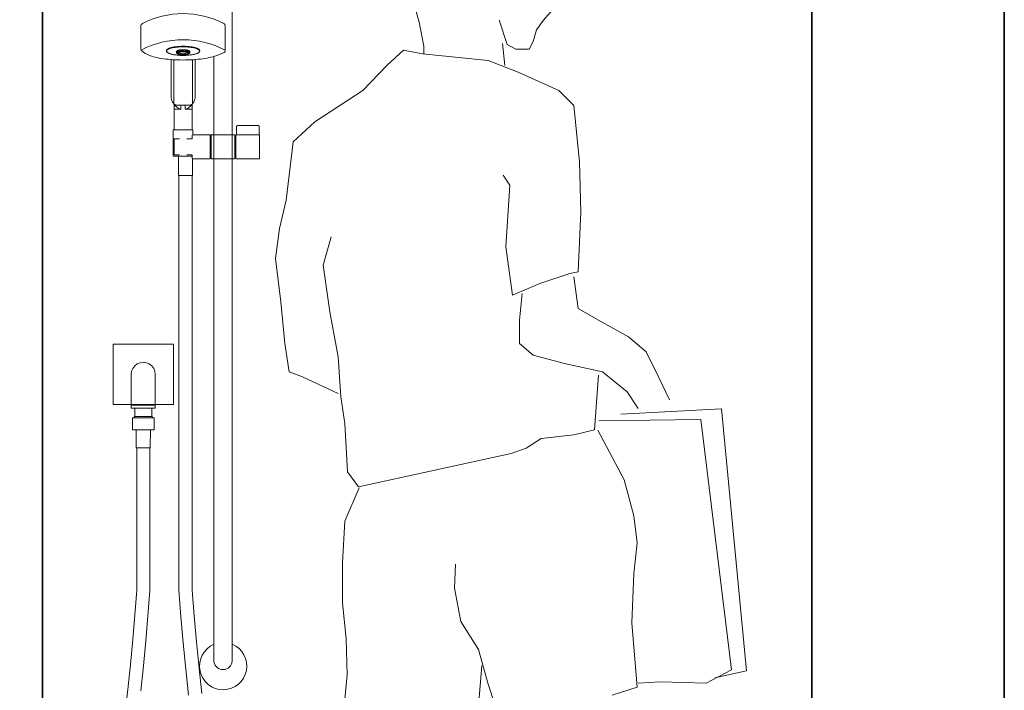
# Model space of a CAD drawing. Units: inches. Extents: x 64 to 1167, y 117 to 939.
# Tile 39 of 56: x 1121 to 1167, y 464 to 496. Entities that reach past the tile are written whole.
import ezdxf

# ---------------------------------------------------------------- set-up
doc = ezdxf.new("R2010")
doc.units = ezdxf.units.IN
doc.header["$MEASUREMENT"] = 0
for name, color, linetype, lineweight in [('A-ENTG', 8, 'Continuous', 18), ('A-FLOR-FIXT', 8, 'Continuous', 18), ('A-SECT', 7, 'Continuous', 35)]:
    doc.layers.add(name, color=color, linetype=linetype, lineweight=lineweight)

# ---------------------------------------------------------------- blocks, each defined once
blk = doc.blocks.new('A$C43851DCA')
at = {"linetype": 'ByBlock'}
for p, q in [((0.0065, 0.059624), (0.006721, 0.058807)), ((0.013179, 0.059624), (0.012552, 0.058897)), ((0.006721, 0.058807), (0.006948, 0.057674)), ((0.010844, 0.057764), (0.01047, 0.058897)), ((0.012552, 0.058897), (0.012215, 0.058446)), ((0.012215, 0.058446), (0.012067, 0.057905)), ((0.006948, 0.057674), (0.006948, 0.057313)), ((0.010733, 0.056772), (0.010623, 0.057809)), ((0.01125, 0.057538), (0.010844, 0.057764)), ((0.012067, 0.057905), (0.011882, 0.057538)), ((0.005999, 0.057487), (0.00523, 0.056785)), ((0.00689, 0.057326), (0.005999, 0.057487)), ((0.009953, 0.057017), (0.00689, 0.057326)), ((0.011882, 0.057538), (0.01125, 0.057538)), ((0.00523, 0.056785), (0.004086, 0.055614)), ((0.011355, 0.05647), (0.009953, 0.057017)), ((0.013269, 0.055614), (0.011355, 0.05647)), ((0.004086, 0.055614), (0.00185, 0.054133)), ((0.01397, 0.054912), (0.013269, 0.055614)), ((0.014223, 0.052266), (0.01397, 0.054912)), ((0.00185, 0.054133), (0.000828, 0.053199)), ((0.000828, 0.053199), (0.000511, 0.050476)), ((0.014292, 0.049929), (0.014223, 0.052266)), ((0.010654, 0.051642), (0.01097, 0.051172)), ((0.01097, 0.051172), (0.010781, 0.048294)), ((0.000511, 0.050476), (0.00019, 0.04915)), ((0.01416, 0.047122), (0.014292, 0.049929)), ((0.00019, 0.04915), (0, 0.047747)), ((0.002615, 0.048758), (0.002235, 0.047438)), ((0.010781, 0.048294), (0.011102, 0.046035)), ((0, 0.047747), (0.000258, 0.045726)), ((0.002235, 0.047438), (0.002552, 0.045256)), ((0.012378, 0.046582), (0.01378, 0.047045)), ((0.01378, 0.047045), (0.01416, 0.047122)), ((0.011102, 0.046035), (0.012378, 0.046582)), ((0.01397, 0.046891), (0.01416, 0.04541)), ((0.011545, 0.046112), (0.011419, 0.044863)), ((0.000258, 0.045726), (0.000448, 0.043775)), ((0.002552, 0.045256), (0.002936, 0.043151)), ((0.01416, 0.04541), (0.015119, 0.044863)), ((0.011419, 0.044863), (0.011419, 0.043775)), ((0.015119, 0.044863), (0.016522, 0.044084)), ((0.000448, 0.043775), (0.000638, 0.042449)), ((0.011419, 0.043775), (0.012056, 0.043228)), ((0.016522, 0.044084), (0.017349, 0.043389)), ((0.017349, 0.043389), (0.017924, 0.042217)), ((0.002936, 0.043151), (0.003063, 0.041284)), ((0.012056, 0.043228), (0.013522, 0.042842)), ((0.000638, 0.042449), (0.001276, 0.042217)), ((0.013522, 0.042842), (0.015309, 0.042449)), ((0.015309, 0.042449), (0.016458, 0.041515)), ((0.001276, 0.042217), (0.002936, 0.041438)), ((0.014929, 0.039726), (0.015119, 0.042294)), ((0.017924, 0.042217), (0.018435, 0.041129)), ((0.016458, 0.041515), (0.01697, 0.040736)), ((0.003063, 0.041284), (0.003253, 0.040035)), ((0.020871, 0.040711), (0.016163, 0.04046)), ((0.022052, 0.028454), (0.020871, 0.040711)), ((0.015135, 0.040151), (0.019901, 0.040209)), ((0.019901, 0.040209), (0.021335, 0.028512)), ((0.003253, 0.040035), (0.003379, 0.037775)), ((0.01397, 0.039494), (0.014929, 0.039726)), ((0.016316, 0.037395), (0.015082, 0.039713)), ((0.01174, 0.03887), (0.012441, 0.039333)), ((0.012441, 0.039333), (0.01397, 0.039494)), ((0.011034, 0.038631), (0.01174, 0.03887)), ((0.003891, 0.037074), (0.011034, 0.038631)), ((0.003379, 0.037775), (0.003891, 0.037074)), ((0.016775, 0.035709), (0.016316, 0.037395)), ((0.003917, 0.037022), (0.003253, 0.035458)), ((0.016927, 0.034453), (0.016775, 0.035709)), ((0.003253, 0.035458), (0.003147, 0.03352)), ((0.016775, 0.033018), (0.016927, 0.034453)), ((0.003147, 0.03352), (0.003147, 0.03164)), ((0.008424, 0.033456), (0.008377, 0.032329)), ((0.016674, 0.030707), (0.016775, 0.033018)), ((0.008377, 0.032329), (0.008683, 0.030765)), ((0.003147, 0.03164), (0.003305, 0.029954)), ((0.008683, 0.030765), (0.0095, 0.029452)), ((0.016927, 0.027701), (0.016674, 0.030707)), ((0.003305, 0.029954), (0.003353, 0.028267)), ((0.0095, 0.029452), (0.009964, 0.027829)), ((0.0095, 0.026825), (0.009658, 0.028705)), ((0.003353, 0.028267), (0.003253, 0.02714)), ((0.021335, 0.028512), (0.020154, 0.027887)), ((0.020565, 0.028138), (0.022052, 0.028454)), ((0.009964, 0.027829), (0.010269, 0.026889)), ((0.015752, 0.027327), (0.016927, 0.027701)), ((0.018003, 0.027952), (0.01698, 0.027887)), ((0.020154, 0.027887), (0.018003, 0.027952))]:
    blk.add_line(p, q, dxfattribs=at)

msp = doc.modelspace()

# ---------------------------------------------------------------- linework, layer by layer
at = {"layer": 'A-FLOR-FIXT'}
for p, q in [((1130.678, 499.898), (1130.678, 490.219)), ((1126.411, 494.238), (1126.411, 495.296)), ((1130.362, 494.172), (1130.362, 495.296)), ((1126.615, 494.023), (1126.467, 494.13)), ((1126.663, 493.994), (1126.615, 494.023)), ((1126.717, 493.967), (1126.663, 493.994)), ((1126.778, 493.94), (1126.717, 493.967)), ((1126.845, 493.914), (1126.778, 493.94)), ((1126.919, 493.89), (1126.845, 493.914)), ((1127.61, 494.153), (1127.612, 494.166)), ((1127.612, 494.141), (1127.61, 494.153)), ((1127.61, 494.128), (1127.612, 494.141)), ((1127.612, 494.115), (1127.61, 494.128)), ((1127.612, 494.166), (1127.616, 494.178)), ((1127.612, 494.141), (1127.616, 494.153)), ((1127.616, 494.102), (1127.612, 494.115)), ((1127.616, 494.178), (1127.624, 494.191)), ((1127.616, 494.153), (1127.624, 494.165)), ((1127.624, 494.09), (1127.616, 494.102)), ((1127.624, 494.191), (1127.635, 494.203)), ((1127.624, 494.165), (1127.635, 494.178)), ((1127.635, 494.078), (1127.624, 494.09)), ((1127.635, 494.103), (1127.625, 494.115)), ((1127.635, 494.203), (1127.648, 494.215)), ((1127.635, 494.178), (1127.648, 494.19)), ((1127.648, 494.091), (1127.635, 494.103)), ((1127.648, 494.066), (1127.635, 494.078)), ((1127.648, 494.215), (1127.665, 494.227)), ((1127.648, 494.19), (1127.665, 494.202)), ((1127.649, 494.09), (1127.648, 494.091)), ((1127.665, 494.054), (1127.648, 494.066)), ((1127.665, 494.227), (1127.684, 494.239)), ((1127.665, 494.202), (1127.684, 494.213)), ((1127.684, 494.042), (1127.665, 494.054)), ((1127.684, 494.239), (1127.706, 494.25)), ((1127.684, 494.213), (1127.706, 494.224)), ((1127.706, 494.031), (1127.684, 494.042)), ((1127.706, 494.25), (1127.731, 494.261)), ((1127.706, 494.224), (1127.731, 494.235)), ((1127.731, 494.02), (1127.706, 494.031)), ((1127.731, 494.261), (1127.759, 494.271)), ((1127.731, 494.235), (1127.759, 494.246)), ((1127.759, 494.01), (1127.731, 494.02)), ((1127.759, 494.271), (1127.788, 494.281)), ((1127.759, 494.246), (1127.788, 494.256)), ((1127.788, 494), (1127.759, 494.01)), ((1127.788, 494.281), (1127.821, 494.291)), ((1127.788, 494.256), (1127.821, 494.265)), ((1127.821, 493.99), (1127.788, 494)), ((1127.821, 494.291), (1127.855, 494.3)), ((1127.821, 494.265), (1127.855, 494.274)), ((1127.855, 493.981), (1127.821, 493.99)), ((1127.855, 494.3), (1127.892, 494.308)), ((1127.855, 494.274), (1127.892, 494.282)), ((1127.892, 493.973), (1127.855, 493.981)), ((1127.892, 494.308), (1127.93, 494.316)), ((1127.892, 494.282), (1127.93, 494.29)), ((1127.93, 493.965), (1127.892, 493.973)), ((1127.93, 494.316), (1127.971, 494.323)), ((1127.93, 494.29), (1127.971, 494.297)), ((1127.971, 493.958), (1127.93, 493.965)), ((1127.971, 494.323), (1128.013, 494.329)), ((1127.971, 494.297), (1128.013, 494.304)), ((1128.013, 493.952), (1127.971, 493.958)), ((1128.013, 494.329), (1128.056, 494.335)), ((1128.013, 494.304), (1128.056, 494.309)), ((1128.056, 493.946), (1128.013, 493.952)), ((1128.056, 494.335), (1128.101, 494.34)), ((1128.056, 494.309), (1128.101, 494.314)), ((1128.101, 493.941), (1128.056, 493.946)), ((1128.076, 494.112), (1128.077, 494.117)), ((1128.077, 494.107), (1128.076, 494.112)), ((1128.077, 494.049), (1128.076, 494.044)), ((1128.076, 494.044), (1128.077, 494.039)), ((1128.077, 494.117), (1128.079, 494.122)), ((1128.079, 494.102), (1128.077, 494.107)), ((1128.079, 494.054), (1128.077, 494.049)), ((1128.077, 494.039), (1128.079, 494.034)), ((1128.079, 494.122), (1128.082, 494.127)), ((1128.079, 494.054), (1128.079, 494.102)), ((1128.082, 494.059), (1128.079, 494.054)), ((1128.079, 494.034), (1128.082, 494.029)), ((1128.082, 494.127), (1128.086, 494.132)), ((1128.086, 494.092), (1128.082, 494.097)), ((1128.086, 494.064), (1128.082, 494.059)), ((1128.082, 494.029), (1128.086, 494.024)), ((1128.086, 494.132), (1128.091, 494.137)), ((1128.091, 494.087), (1128.086, 494.092)), ((1128.091, 494.069), (1128.086, 494.064)), ((1128.086, 494.024), (1128.091, 494.019)), ((1128.091, 494.137), (1128.098, 494.142)), ((1128.098, 494.083), (1128.091, 494.087)), ((1128.091, 494.069), (1128.098, 494.074)), ((1128.091, 494.019), (1128.098, 494.015)), ((1128.098, 494.142), (1128.106, 494.146)), ((1128.106, 494.078), (1128.098, 494.083)), ((1128.098, 494.074), (1128.106, 494.078)), ((1128.098, 494.015), (1128.106, 494.01)), ((1128.101, 494.34), (1128.147, 494.344)), ((1128.101, 494.314), (1128.147, 494.319)), ((1128.147, 493.937), (1128.101, 493.941)), ((1128.106, 494.146), (1128.114, 494.151)), ((1128.106, 494.078), (1128.111, 494.081)), ((1128.111, 494.075), (1128.106, 494.078)), ((1128.106, 494.01), (1128.114, 494.005)), ((1128.111, 494.081), (1128.114, 494.083)), ((1128.111, 494.081), (1128.111, 494.075)), ((1128.114, 494.074), (1128.111, 494.075)), ((1128.111, 494.075), (1128.111, 494.062)), ((1128.111, 494.058), (1128.114, 494.053)), ((1128.111, 494.044), (1128.112, 494.049)), ((1128.112, 494.04), (1128.111, 494.044)), ((1128.112, 494.049), (1128.114, 494.053)), ((1128.114, 494.035), (1128.112, 494.04)), ((1128.114, 494.151), (1128.124, 494.155)), ((1128.116, 494.126), (1128.114, 494.123)), ((1128.116, 494.115), (1128.114, 494.112)), ((1128.114, 494.092), (1128.116, 494.089)), ((1128.114, 494.083), (1128.12, 494.084)), ((1128.124, 494.069), (1128.114, 494.074)), ((1128.114, 494.053), (1128.116, 494.057)), ((1128.116, 494.031), (1128.114, 494.035)), ((1128.114, 494.005), (1128.124, 494.001)), ((1128.12, 494.13), (1128.116, 494.126)), ((1128.12, 494.12), (1128.116, 494.115)), ((1128.116, 494.089), (1128.12, 494.084)), ((1128.116, 494.057), (1128.12, 494.062)), ((1128.12, 494.026), (1128.116, 494.031)), ((1128.125, 494.134), (1128.12, 494.13)), ((1128.125, 494.124), (1128.12, 494.12)), ((1128.12, 494.084), (1128.124, 494.087)), ((1128.12, 494.084), (1128.125, 494.08)), ((1128.12, 494.062), (1128.125, 494.066)), ((1128.125, 494.022), (1128.12, 494.026)), ((1128.124, 494.155), (1128.135, 494.159)), ((1128.124, 494.087), (1128.135, 494.091)), ((1128.127, 494.068), (1128.124, 494.069)), ((1128.124, 494.001), (1128.135, 493.997)), ((1128.131, 494.138), (1128.125, 494.134)), ((1128.131, 494.128), (1128.125, 494.124)), ((1128.125, 494.08), (1128.131, 494.076)), ((1128.125, 494.066), (1128.127, 494.068)), ((1128.131, 494.018), (1128.125, 494.022)), ((1128.127, 494.068), (1128.131, 494.07)), ((1128.135, 494.065), (1128.127, 494.068)), ((1128.135, 494.141), (1128.131, 494.138)), ((1128.135, 494.131), (1128.131, 494.128)), ((1128.131, 494.076), (1128.135, 494.073)), ((1128.131, 494.07), (1128.135, 494.073)), ((1128.138, 494.014), (1128.131, 494.018)), ((1128.135, 494.159), (1128.147, 494.163)), ((1128.135, 494.091), (1128.147, 494.095)), ((1128.135, 494.073), (1128.138, 494.074)), ((1128.135, 494.073), (1128.138, 494.072)), ((1128.138, 494.064), (1128.135, 494.065)), ((1128.135, 493.997), (1128.147, 493.993)), ((1128.138, 494.074), (1128.145, 494.078)), ((1128.138, 494.072), (1128.145, 494.068)), ((1128.145, 494.01), (1128.138, 494.014)), ((1128.145, 494.078), (1128.154, 494.082)), ((1128.145, 494.068), (1128.154, 494.064)), ((1128.147, 494.061), (1128.145, 494.062)), ((1128.154, 494.006), (1128.145, 494.01)), ((1128.147, 494.344), (1128.193, 494.348)), ((1128.147, 494.319), (1128.193, 494.322)), ((1128.147, 494.163), (1128.16, 494.167)), ((1128.154, 494.15), (1128.147, 494.147)), ((1128.154, 494.14), (1128.147, 494.137)), ((1128.16, 494.099), (1128.147, 494.095)), ((1128.16, 494.057), (1128.147, 494.061)), ((1128.147, 493.993), (1128.16, 493.989)), ((1128.193, 493.933), (1128.147, 493.937)), ((1128.16, 494.153), (1128.154, 494.15)), ((1128.16, 494.142), (1128.154, 494.14)), ((1128.154, 494.082), (1128.164, 494.086)), ((1128.154, 494.064), (1128.164, 494.06)), ((1128.164, 494.002), (1128.154, 494.006)), ((1128.16, 494.167), (1128.174, 494.171)), ((1128.174, 494.103), (1128.16, 494.099)), ((1128.164, 494.056), (1128.16, 494.057)), ((1128.16, 493.989), (1128.174, 493.986)), ((1128.164, 494.086), (1128.174, 494.089)), ((1128.164, 494.06), (1128.174, 494.057)), ((1128.174, 493.999), (1128.164, 494.002)), ((1128.174, 494.171), (1128.189, 494.174)), ((1128.186, 494.161), (1128.174, 494.158)), ((1128.186, 494.151), (1128.174, 494.147)), ((1128.189, 494.106), (1128.174, 494.103)), ((1128.174, 494.089), (1128.186, 494.093)), ((1128.174, 494.057), (1128.186, 494.053)), ((1128.186, 494.051), (1128.174, 494.054)), ((1128.186, 493.995), (1128.174, 493.999)), ((1128.174, 493.986), (1128.189, 493.982)), ((1128.189, 494.162), (1128.186, 494.161)), ((1128.189, 494.151), (1128.186, 494.151)), ((1128.186, 494.093), (1128.198, 494.096)), ((1128.186, 494.053), (1128.198, 494.05)), ((1128.198, 493.992), (1128.186, 493.995)), ((1128.189, 494.174), (1128.204, 494.177)), ((1128.204, 494.109), (1128.189, 494.106)), ((1128.189, 493.982), (1128.204, 493.979)), ((1128.193, 494.348), (1128.241, 494.35)), ((1128.193, 494.322), (1128.241, 494.325)), ((1128.241, 493.93), (1128.193, 493.933)), ((1128.198, 494.096), (1128.211, 494.099)), ((1128.198, 494.05), (1128.204, 494.047)), ((1128.204, 494.047), (1128.198, 494.048)), ((1128.211, 493.989), (1128.198, 493.992)), ((1128.204, 494.177), (1128.22, 494.18)), ((1128.211, 494.167), (1128.204, 494.165)), ((1128.211, 494.157), (1128.204, 494.155)), ((1128.22, 494.112), (1128.204, 494.109)), ((1128.204, 494.047), (1128.211, 494.047)), ((1128.204, 493.979), (1128.22, 493.976)), ((1128.22, 494.169), (1128.211, 494.167)), ((1128.22, 494.159), (1128.211, 494.157)), ((1128.211, 494.099), (1128.225, 494.102)), ((1128.211, 494.047), (1128.22, 494.044)), ((1128.225, 493.986), (1128.211, 493.989)), ((1128.22, 494.18), (1128.237, 494.183)), ((1128.237, 494.114), (1128.22, 494.112)), ((1128.225, 494.044), (1128.22, 494.044)), ((1128.22, 493.976), (1128.237, 493.974)), ((1128.225, 494.102), (1128.239, 494.104)), ((1128.225, 494.044), (1128.239, 494.042)), ((1128.239, 493.984), (1128.225, 493.986)), ((1128.237, 494.183), (1128.254, 494.185)), ((1128.254, 494.117), (1128.237, 494.114)), ((1128.237, 493.974), (1128.254, 493.971)), ((1128.239, 494.104), (1128.254, 494.106)), ((1128.239, 494.042), (1128.254, 494.04)), ((1128.254, 493.982), (1128.239, 493.984)), ((1128.241, 494.35), (1128.289, 494.352)), ((1128.241, 494.325), (1128.289, 494.327)), ((1128.289, 493.928), (1128.241, 493.93)), ((1128.254, 494.185), (1128.272, 494.187)), ((1128.269, 494.177), (1128.254, 494.175)), ((1128.269, 494.166), (1128.254, 494.164)), ((1128.272, 494.119), (1128.254, 494.117)), ((1128.254, 494.106), (1128.269, 494.109)), ((1128.254, 494.04), (1128.269, 494.038)), ((1128.269, 493.98), (1128.254, 493.982)), ((1128.254, 493.971), (1128.272, 493.969)), ((1128.272, 494.177), (1128.269, 494.177)), ((1128.272, 494.167), (1128.269, 494.166)), ((1128.269, 494.109), (1128.285, 494.11)), ((1128.269, 494.038), (1128.285, 494.036)), ((1128.285, 493.978), (1128.269, 493.98)), ((1128.272, 494.187), (1128.291, 494.189)), ((1128.291, 494.12), (1128.272, 494.119)), ((1128.272, 493.969), (1128.291, 493.968)), ((1128.285, 494.11), (1128.301, 494.112)), ((1128.285, 494.036), (1128.301, 494.034)), ((1128.301, 493.976), (1128.285, 493.978)), ((1128.289, 494.352), (1128.338, 494.354)), ((1128.289, 494.327), (1128.338, 494.328)), ((1128.338, 493.927), (1128.289, 493.928)), ((1128.291, 494.189), (1128.309, 494.19)), ((1128.301, 494.18), (1128.291, 494.179)), ((1128.301, 494.17), (1128.291, 494.169)), ((1128.309, 494.122), (1128.291, 494.12)), ((1128.291, 493.968), (1128.309, 493.966)), ((1128.309, 494.181), (1128.301, 494.18)), ((1128.309, 494.17), (1128.301, 494.17)), ((1128.301, 494.112), (1128.318, 494.113)), ((1128.301, 494.034), (1128.318, 494.033)), ((1128.318, 493.975), (1128.301, 493.976)), ((1128.309, 494.19), (1128.328, 494.191)), ((1128.328, 494.123), (1128.309, 494.122)), ((1128.309, 493.966), (1128.328, 493.965)), ((1128.318, 494.113), (1128.335, 494.114)), ((1128.318, 494.033), (1128.335, 494.032)), ((1128.335, 493.974), (1128.318, 493.975)), ((1128.328, 494.191), (1128.348, 494.192)), ((1128.348, 494.124), (1128.328, 494.123)), ((1128.328, 493.965), (1128.348, 493.964)), ((1128.335, 494.114), (1128.352, 494.115)), ((1128.335, 494.032), (1128.352, 494.031)), ((1128.352, 493.973), (1128.335, 493.974)), ((1128.338, 494.354), (1128.386, 494.354)), ((1128.338, 494.328), (1128.386, 494.328)), ((1128.386, 493.927), (1128.338, 493.927)), ((1128.348, 494.192), (1128.367, 494.192)), ((1128.352, 494.183), (1128.348, 494.183)), ((1128.352, 494.173), (1128.348, 494.172)), ((1128.367, 494.124), (1128.348, 494.124)), ((1128.348, 493.964), (1128.367, 493.964)), ((1128.367, 494.183), (1128.352, 494.183)), ((1128.367, 494.173), (1128.352, 494.173)), ((1128.352, 494.115), (1128.369, 494.115)), ((1128.352, 494.031), (1128.369, 494.031)), ((1128.369, 493.973), (1128.352, 493.973)), ((1128.367, 494.192), (1128.386, 494.193)), ((1128.386, 494.124), (1128.367, 494.124)), ((1128.367, 493.964), (1128.386, 493.964)), ((1128.369, 494.115), (1128.386, 494.115)), ((1128.369, 494.031), (1128.386, 494.031)), ((1128.386, 493.973), (1128.369, 493.973)), ((1128.386, 494.354), (1128.435, 494.354)), ((1128.386, 494.328), (1128.435, 494.328)), ((1128.386, 494.193), (1128.406, 494.192)), ((1128.406, 494.124), (1128.386, 494.124)), ((1128.386, 494.115), (1128.404, 494.115)), ((1128.386, 494.031), (1128.404, 494.031)), ((1128.404, 493.973), (1128.386, 493.973)), ((1128.386, 493.964), (1128.406, 493.964)), ((1128.435, 493.927), (1128.386, 493.927)), ((1128.404, 494.115), (1128.421, 494.115)), ((1128.404, 494.031), (1128.421, 494.031)), ((1128.421, 493.973), (1128.404, 493.973)), ((1128.406, 494.192), (1128.425, 494.192)), ((1128.421, 494.183), (1128.406, 494.183)), ((1128.421, 494.173), (1128.406, 494.173)), ((1128.425, 494.124), (1128.406, 494.124)), ((1128.406, 493.964), (1128.425, 493.964)), ((1128.425, 494.183), (1128.421, 494.183)), ((1128.425, 494.172), (1128.421, 494.173)), ((1128.421, 494.115), (1128.438, 494.114)), ((1128.421, 494.031), (1128.438, 494.032)), ((1128.438, 493.974), (1128.421, 493.973)), ((1128.425, 494.192), (1128.445, 494.191)), ((1128.445, 494.123), (1128.425, 494.124)), ((1128.425, 493.964), (1128.445, 493.965)), ((1128.435, 494.354), (1128.484, 494.352)), ((1128.435, 494.328), (1128.484, 494.327)), ((1128.484, 493.928), (1128.435, 493.927)), ((1128.438, 494.114), (1128.455, 494.113)), ((1128.438, 494.032), (1128.455, 494.033)), ((1128.455, 493.975), (1128.438, 493.974)), ((1128.445, 494.191), (1128.464, 494.19)), ((1128.464, 494.122), (1128.445, 494.123)), ((1128.445, 493.965), (1128.464, 493.966)), ((1128.455, 494.113), (1128.471, 494.112)), ((1128.455, 494.033), (1128.471, 494.034)), ((1128.471, 493.976), (1128.455, 493.975)), ((1128.464, 494.19), (1128.482, 494.189)), ((1128.471, 494.18), (1128.464, 494.181)), ((1128.471, 494.17), (1128.464, 494.17)), ((1128.464, 494.122), (1128.482, 494.12)), ((1128.464, 493.966), (1128.482, 493.968)), ((1128.482, 494.179), (1128.471, 494.18)), ((1128.482, 494.169), (1128.471, 494.17)), ((1128.471, 494.112), (1128.488, 494.11)), ((1128.471, 494.034), (1128.488, 494.036)), ((1128.488, 493.978), (1128.471, 493.976)), ((1128.482, 494.189), (1128.501, 494.187)), ((1128.482, 494.12), (1128.501, 494.119)), ((1128.482, 493.968), (1128.501, 493.969)), ((1128.484, 494.352), (1128.532, 494.35)), ((1128.484, 494.327), (1128.532, 494.325)), ((1128.532, 493.93), (1128.484, 493.928)), ((1128.488, 494.11), (1128.504, 494.109)), ((1128.488, 494.036), (1128.504, 494.038)), ((1128.504, 493.98), (1128.488, 493.978)), ((1128.501, 494.187), (1128.519, 494.185)), ((1128.501, 494.119), (1128.519, 494.117)), ((1128.501, 493.969), (1128.519, 493.971)), ((1128.504, 494.109), (1128.519, 494.106)), ((1128.504, 494.038), (1128.519, 494.04)), ((1128.519, 493.982), (1128.504, 493.98)), ((1128.519, 494.185), (1128.536, 494.183)), ((1128.534, 494.172), (1128.519, 494.175)), ((1128.534, 494.162), (1128.519, 494.164)), ((1128.519, 494.117), (1128.536, 494.114)), ((1128.519, 494.106), (1128.534, 494.104)), ((1128.519, 494.04), (1128.534, 494.042)), ((1128.534, 493.984), (1128.519, 493.982)), ((1128.519, 493.971), (1128.536, 493.974)), ((1128.532, 494.35), (1128.579, 494.348)), ((1128.532, 494.325), (1128.579, 494.322)), ((1128.579, 493.933), (1128.532, 493.93)), ((1128.536, 494.172), (1128.534, 494.172)), ((1128.536, 494.162), (1128.534, 494.162)), ((1128.534, 494.104), (1128.548, 494.102)), ((1128.534, 494.042), (1128.548, 494.044)), ((1128.548, 493.986), (1128.534, 493.984)), ((1128.536, 494.183), (1128.553, 494.18)), ((1128.536, 494.114), (1128.553, 494.112)), ((1128.536, 493.974), (1128.553, 493.976)), ((1128.548, 494.102), (1128.562, 494.099)), ((1128.553, 494.044), (1128.548, 494.044)), ((1128.562, 493.989), (1128.548, 493.986)), ((1128.553, 494.18), (1128.569, 494.177)), ((1128.562, 494.167), (1128.553, 494.169)), ((1128.562, 494.157), (1128.553, 494.159)), ((1128.553, 494.112), (1128.569, 494.109)), ((1128.562, 494.047), (1128.553, 494.044)), ((1128.553, 493.976), (1128.569, 493.979)), ((1128.569, 494.165), (1128.562, 494.167)), ((1128.569, 494.155), (1128.562, 494.157)), ((1128.562, 494.099), (1128.575, 494.096)), ((1128.562, 494.047), (1128.575, 494.05)), ((1128.575, 493.992), (1128.562, 493.989)), ((1128.569, 494.177), (1128.584, 494.174)), ((1128.569, 494.109), (1128.584, 494.106)), ((1128.569, 493.979), (1128.584, 493.982)), ((1128.575, 494.096), (1128.587, 494.093)), ((1128.575, 494.05), (1128.587, 494.053)), ((1128.584, 494.05), (1128.575, 494.048)), ((1128.587, 493.995), (1128.575, 493.992)), ((1128.579, 494.348), (1128.626, 494.344)), ((1128.579, 494.322), (1128.626, 494.319)), ((1128.626, 493.937), (1128.579, 493.933)), ((1128.584, 494.174), (1128.599, 494.171)), ((1128.587, 494.161), (1128.584, 494.162)), ((1128.587, 494.151), (1128.584, 494.151)), ((1128.584, 494.106), (1128.599, 494.103)), ((1128.598, 494.054), (1128.584, 494.05)), ((1128.584, 493.982), (1128.599, 493.986)), ((1128.598, 494.158), (1128.587, 494.161)), ((1128.598, 494.147), (1128.587, 494.151)), ((1128.587, 494.093), (1128.598, 494.089)), ((1128.587, 494.053), (1128.598, 494.057)), ((1128.598, 493.999), (1128.587, 493.995)), ((1128.598, 494.089), (1128.609, 494.086)), ((1128.598, 494.057), (1128.609, 494.06)), ((1128.609, 494.002), (1128.598, 493.999)), ((1128.599, 494.171), (1128.613, 494.167)), ((1128.599, 494.103), (1128.613, 494.099)), ((1128.599, 493.986), (1128.613, 493.989)), ((1128.609, 494.086), (1128.619, 494.082)), ((1128.609, 494.06), (1128.619, 494.064)), ((1128.613, 494.057), (1128.609, 494.056)), ((1128.619, 494.006), (1128.609, 494.002)), ((1128.613, 494.167), (1128.626, 494.163)), ((1128.619, 494.15), (1128.613, 494.153)), ((1128.619, 494.14), (1128.613, 494.142)), ((1128.613, 494.099), (1128.626, 494.095)), ((1128.626, 494.061), (1128.613, 494.057)), ((1128.613, 493.989), (1128.626, 493.993)), ((1128.626, 494.147), (1128.619, 494.15)), ((1128.626, 494.137), (1128.619, 494.14)), ((1128.619, 494.082), (1128.627, 494.078)), ((1128.619, 494.064), (1128.627, 494.068)), ((1128.627, 494.01), (1128.619, 494.006)), ((1128.626, 494.344), (1128.672, 494.34)), ((1128.626, 494.319), (1128.672, 494.314)), ((1128.626, 494.163), (1128.638, 494.159)), ((1128.626, 494.095), (1128.638, 494.091)), ((1128.627, 494.062), (1128.626, 494.061)), ((1128.626, 493.993), (1128.638, 493.997)), ((1128.672, 493.941), (1128.626, 493.937)), ((1128.627, 494.078), (1128.635, 494.074)), ((1128.627, 494.068), (1128.635, 494.072)), ((1128.635, 494.014), (1128.627, 494.01)), ((1128.635, 494.074), (1128.638, 494.073)), ((1128.635, 494.072), (1128.638, 494.073)), ((1128.638, 494.065), (1128.635, 494.064)), ((1128.642, 494.018), (1128.635, 494.014)), ((1128.638, 494.159), (1128.648, 494.155)), ((1128.642, 494.138), (1128.638, 494.141)), ((1128.642, 494.128), (1128.638, 494.131)), ((1128.638, 494.091), (1128.648, 494.087)), ((1128.638, 494.073), (1128.642, 494.076)), ((1128.638, 494.073), (1128.642, 494.07)), ((1128.645, 494.068), (1128.638, 494.065)), ((1128.638, 493.997), (1128.648, 494.001)), ((1128.648, 494.134), (1128.642, 494.138)), ((1128.648, 494.124), (1128.642, 494.128)), ((1128.642, 494.076), (1128.648, 494.08)), ((1128.642, 494.07), (1128.645, 494.068)), ((1128.648, 494.022), (1128.642, 494.018)), ((1128.648, 494.069), (1128.645, 494.068)), ((1128.645, 494.068), (1128.648, 494.066)), ((1128.648, 494.155), (1128.658, 494.151)), ((1128.648, 494.087), (1128.653, 494.084)), ((1128.648, 494.08), (1128.653, 494.084)), ((1128.657, 494.073), (1128.648, 494.069)), ((1128.648, 494.066), (1128.653, 494.062)), ((1128.653, 494.026), (1128.648, 494.022)), ((1128.648, 494.001), (1128.658, 494.005)), ((1128.653, 494.084), (1128.658, 494.083)), ((1128.653, 494.062), (1128.657, 494.057)), ((1128.657, 494.031), (1128.653, 494.026)), ((1128.657, 494.057), (1128.659, 494.053)), ((1128.659, 494.035), (1128.657, 494.031)), ((1128.658, 494.151), (1128.667, 494.146)), ((1128.659, 494.121), (1128.658, 494.123)), ((1128.659, 494.111), (1128.658, 494.112)), ((1128.658, 494.092), (1128.659, 494.093)), ((1128.661, 494.081), (1128.658, 494.092)), ((1128.658, 494.083), (1128.661, 494.081)), ((1128.658, 494.005), (1128.667, 494.01)), ((1128.661, 494.117), (1128.659, 494.121)), ((1128.661, 494.108), (1128.659, 494.111)), ((1128.659, 494.093), (1128.661, 494.098)), ((1128.661, 494.075), (1128.659, 494.074)), ((1128.659, 494.053), (1128.661, 494.058)), ((1128.659, 494.053), (1128.661, 494.049)), ((1128.661, 494.04), (1128.659, 494.035)), ((1128.661, 494.112), (1128.661, 494.117)), ((1128.661, 494.108), (1128.661, 494.112)), ((1128.661, 494.106), (1128.661, 494.108)), ((1128.661, 494.102), (1128.661, 494.106)), ((1128.661, 494.098), (1128.661, 494.102)), ((1128.661, 494.062), (1128.661, 494.075)), ((1128.661, 494.049), (1128.661, 494.044)), ((1128.661, 494.044), (1128.661, 494.04)), ((1128.661, 494.081), (1128.667, 494.078)), ((1128.661, 494.075), (1128.661, 494.081)), ((1128.667, 494.078), (1128.661, 494.075)), ((1128.667, 494.146), (1128.675, 494.142)), ((1128.675, 494.083), (1128.667, 494.078)), ((1128.667, 494.078), (1128.675, 494.074)), ((1128.675, 494.015), (1128.667, 494.01)), ((1128.672, 494.34), (1128.717, 494.335)), ((1128.672, 494.314), (1128.717, 494.309)), ((1128.717, 493.946), (1128.672, 493.941)), ((1128.675, 494.142), (1128.682, 494.137)), ((1128.682, 494.087), (1128.675, 494.083)), ((1128.675, 494.074), (1128.682, 494.069)), ((1128.682, 494.019), (1128.675, 494.015)), ((1128.682, 494.137), (1128.687, 494.132)), ((1128.682, 494.069), (1128.687, 494.064)), ((1128.687, 494.024), (1128.682, 494.019)), ((1128.687, 494.132), (1128.691, 494.127)), ((1128.691, 494.097), (1128.687, 494.092)), ((1128.687, 494.064), (1128.691, 494.059)), ((1128.691, 494.029), (1128.687, 494.024)), ((1128.691, 494.127), (1128.694, 494.122)), ((1128.694, 494.102), (1128.691, 494.097)), ((1128.694, 494.054), (1128.691, 494.059)), ((1128.694, 494.034), (1128.691, 494.029)), ((1128.694, 494.122), (1128.696, 494.117)), ((1128.696, 494.107), (1128.694, 494.102)), ((1128.694, 494.054), (1128.694, 494.102)), ((1128.696, 494.049), (1128.694, 494.054)), ((1128.696, 494.039), (1128.694, 494.034)), ((1128.696, 494.117), (1128.697, 494.112)), ((1128.697, 494.112), (1128.696, 494.107)), ((1128.696, 494.049), (1128.697, 494.044)), ((1128.697, 494.044), (1128.696, 494.039)), ((1128.717, 494.335), (1128.76, 494.329)), ((1128.717, 494.309), (1128.76, 494.304)), ((1128.76, 493.952), (1128.717, 493.946)), ((1128.76, 494.329), (1128.802, 494.323)), ((1128.76, 494.304), (1128.802, 494.297)), ((1128.802, 493.958), (1128.76, 493.952)), ((1128.802, 494.323), (1128.843, 494.316)), ((1128.802, 494.297), (1128.843, 494.29)), ((1128.843, 493.965), (1128.802, 493.958)), ((1128.843, 494.316), (1128.881, 494.308)), ((1128.843, 494.29), (1128.881, 494.282)), ((1128.881, 493.973), (1128.843, 493.965)), ((1128.881, 494.308), (1128.918, 494.3)), ((1128.881, 494.282), (1128.918, 494.274)), ((1128.918, 493.981), (1128.881, 493.973)), ((1128.918, 494.3), (1128.952, 494.291)), ((1128.918, 494.274), (1128.952, 494.265)), ((1128.952, 493.99), (1128.918, 493.981)), ((1128.952, 494.291), (1128.984, 494.281)), ((1128.952, 494.265), (1128.984, 494.256)), ((1128.984, 494), (1128.952, 493.99)), ((1128.984, 494.281), (1129.014, 494.271)), ((1128.984, 494.256), (1129.014, 494.246)), ((1129.014, 494.01), (1128.984, 494)), ((1129.014, 494.271), (1129.042, 494.261)), ((1129.014, 494.246), (1129.042, 494.235)), ((1129.042, 494.02), (1129.014, 494.01)), ((1129.042, 494.261), (1129.066, 494.25)), ((1129.042, 494.235), (1129.066, 494.224)), ((1129.066, 494.031), (1129.042, 494.02)), ((1129.066, 494.25), (1129.089, 494.239)), ((1129.066, 494.224), (1129.089, 494.213)), ((1129.089, 494.042), (1129.066, 494.031)), ((1129.089, 494.239), (1129.108, 494.227)), ((1129.089, 494.213), (1129.108, 494.202)), ((1129.108, 494.054), (1129.089, 494.042)), ((1129.108, 494.227), (1129.124, 494.215)), ((1129.108, 494.202), (1129.124, 494.19)), ((1129.124, 494.066), (1129.108, 494.054)), ((1129.124, 494.215), (1129.138, 494.203)), ((1129.124, 494.19), (1129.138, 494.178)), ((1129.138, 494.078), (1129.124, 494.066)), ((1129.138, 494.103), (1129.137, 494.102)), ((1129.138, 494.203), (1129.149, 494.191)), ((1129.138, 494.178), (1129.149, 494.165)), ((1129.148, 494.115), (1129.138, 494.103)), ((1129.149, 494.09), (1129.138, 494.078)), ((1129.149, 494.191), (1129.156, 494.178)), ((1129.149, 494.165), (1129.156, 494.153)), ((1129.156, 494.102), (1129.149, 494.09)), ((1129.156, 494.178), (1129.161, 494.166)), ((1129.156, 494.153), (1129.161, 494.14)), ((1129.161, 494.115), (1129.156, 494.102)), ((1129.161, 494.166), (1129.162, 494.153)), ((1129.162, 494.153), (1129.161, 494.14)), ((1129.161, 494.14), (1129.162, 494.128)), ((1129.162, 494.128), (1129.161, 494.115)), ((1129.927, 493.914), (1129.854, 493.89)), ((1130.276, 494.047), (1129.927, 493.914)), ((1126.998, 493.867), (1126.919, 493.89)), ((1127.082, 493.845), (1126.998, 493.867)), ((1127.172, 493.824), (1127.082, 493.845)), ((1127.267, 493.805), (1127.172, 493.824)), ((1127.366, 493.788), (1127.267, 493.805)), ((1127.469, 493.772), (1127.366, 493.788)), ((1127.575, 493.758), (1127.469, 493.772)), ((1127.685, 493.746), (1127.575, 493.758)), ((1127.798, 493.735), (1127.685, 493.746)), ((1127.822, 493.734), (1127.798, 493.735)), ((1127.822, 492.016), (1127.822, 493.734)), ((1127.913, 493.727), (1127.822, 493.734)), ((1127.946, 493.725), (1127.913, 493.727)), ((1127.946, 491.666), (1127.946, 493.725)), ((1127.951, 493.725), (1127.946, 493.725)), ((1127.956, 493.724), (1127.951, 493.725)), ((1127.961, 493.724), (1127.956, 493.724)), ((1127.966, 493.724), (1127.961, 493.724)), ((1127.973, 493.723), (1127.966, 493.724)), ((1127.975, 493.723), (1127.973, 493.723)), ((1127.98, 493.723), (1127.975, 493.723)), ((1127.986, 493.722), (1127.98, 493.723)), ((1127.993, 493.722), (1127.986, 493.722)), ((1128.001, 493.722), (1127.993, 493.722)), ((1128.008, 493.721), (1128.001, 493.722)), ((1128.015, 493.721), (1128.008, 493.721)), ((1128.023, 493.72), (1128.015, 493.721)), ((1128.029, 493.72), (1128.023, 493.72)), ((1128.031, 493.72), (1128.029, 493.72)), ((1128.039, 493.72), (1128.031, 493.72)), ((1128.046, 493.719), (1128.039, 493.72)), ((1128.054, 493.719), (1128.046, 493.719)), ((1128.062, 493.719), (1128.054, 493.719)), ((1128.07, 493.718), (1128.062, 493.719)), ((1128.077, 493.718), (1128.07, 493.718)), ((1128.085, 493.718), (1128.077, 493.718)), ((1128.092, 493.717), (1128.085, 493.718)), ((1128.099, 493.717), (1128.092, 493.717)), ((1128.106, 493.717), (1128.099, 493.717)), ((1128.148, 493.715), (1128.106, 493.717)), ((1128.267, 493.712), (1128.148, 493.715)), ((1128.386, 493.711), (1128.267, 493.712)), ((1128.506, 493.712), (1128.386, 493.711)), ((1128.625, 493.715), (1128.506, 493.712)), ((1128.667, 493.717), (1128.625, 493.715)), ((1128.674, 493.717), (1128.667, 493.717)), ((1128.681, 493.717), (1128.674, 493.717)), ((1128.688, 493.718), (1128.681, 493.717)), ((1128.696, 493.718), (1128.688, 493.718)), ((1128.703, 493.718), (1128.696, 493.718)), ((1128.711, 493.719), (1128.703, 493.718)), ((1128.719, 493.719), (1128.711, 493.719)), ((1128.726, 493.719), (1128.719, 493.719)), ((1128.734, 493.72), (1128.726, 493.719)), ((1128.742, 493.72), (1128.734, 493.72)), ((1128.743, 493.72), (1128.742, 493.72)), ((1128.75, 493.72), (1128.743, 493.72)), ((1128.757, 493.721), (1128.75, 493.72)), ((1128.765, 493.721), (1128.757, 493.721)), ((1128.772, 493.722), (1128.765, 493.721)), ((1128.78, 493.722), (1128.772, 493.722)), ((1128.786, 493.722), (1128.78, 493.722)), ((1128.793, 493.723), (1128.786, 493.722)), ((1128.798, 493.723), (1128.793, 493.723)), ((1128.806, 493.724), (1128.798, 493.723)), ((1128.812, 493.724), (1128.806, 493.724)), ((1128.817, 493.724), (1128.812, 493.724)), ((1128.822, 493.725), (1128.817, 493.724)), ((1128.827, 493.725), (1128.822, 493.725)), ((1128.86, 493.727), (1128.827, 493.725)), ((1128.827, 493.725), (1128.827, 491.658)), ((1128.951, 493.734), (1128.86, 493.727)), ((1128.975, 493.735), (1128.951, 493.734)), ((1128.951, 492.016), (1128.951, 493.734)), ((1129.088, 493.746), (1128.975, 493.735)), ((1129.197, 493.758), (1129.088, 493.746)), ((1129.304, 493.772), (1129.197, 493.758)), ((1129.407, 493.788), (1129.304, 493.772)), ((1129.506, 493.805), (1129.407, 493.788)), ((1129.601, 493.824), (1129.506, 493.805)), ((1129.69, 493.845), (1129.601, 493.824)), ((1129.775, 493.867), (1129.69, 493.845)), ((1129.832, 493.883), (1129.775, 493.867)), ((1129.854, 493.89), (1129.832, 493.883)), ((1129.832, 490.219), (1129.832, 493.883)), ((1127.826, 491.946), (1127.822, 492.016)), ((1127.84, 491.876), (1127.826, 491.946)), ((1127.862, 491.809), (1127.84, 491.876)), ((1127.892, 491.745), (1127.862, 491.809)), ((1127.93, 491.685), (1127.892, 491.745)), ((1127.946, 491.666), (1127.93, 491.685)), ((1127.946, 491.658), (1127.946, 491.666)), ((1127.951, 491.66), (1127.946, 491.666)), ((1127.951, 491.654), (1127.946, 491.658)), ((1127.956, 491.654), (1127.951, 491.66)), ((1127.956, 491.65), (1127.951, 491.654)), ((1127.961, 491.647), (1127.956, 491.654)), ((1127.975, 491.631), (1127.956, 491.65)), ((1127.961, 491.646), (1127.961, 491.647)), ((1127.964, 491.644), (1127.961, 491.646)), ((1127.967, 491.641), (1127.964, 491.644)), ((1127.964, 491.644), (1127.964, 491.406)), ((1127.967, 491.633), (1127.966, 491.642)), ((1127.972, 491.639), (1127.967, 491.641)), ((1127.967, 491.633), (1127.967, 491.574)), ((1127.973, 491.637), (1127.972, 491.639)), ((1127.973, 491.634), (1127.973, 491.637)), ((1127.98, 491.634), (1127.973, 491.637)), ((1127.975, 491.631), (1127.973, 491.634)), ((1127.975, 491.631), (1127.977, 491.612)), ((1127.977, 491.612), (1127.994, 491.568)), ((1127.986, 491.63), (1127.98, 491.634)), ((1127.993, 491.626), (1127.986, 491.63)), ((1128.001, 491.623), (1127.993, 491.626)), ((1128.008, 491.619), (1128.001, 491.623)), ((1128.001, 491.623), (1128.003, 491.614)), ((1128.003, 491.614), (1128.029, 491.572)), ((1128.015, 491.616), (1128.008, 491.619)), ((1128.023, 491.613), (1128.015, 491.616)), ((1128.031, 491.61), (1128.023, 491.613)), ((1128.039, 491.607), (1128.031, 491.61)), ((1128.046, 491.605), (1128.039, 491.607)), ((1128.054, 491.603), (1128.046, 491.605)), ((1128.726, 491.605), (1128.719, 491.603)), ((1128.734, 491.607), (1128.726, 491.605)), ((1128.742, 491.61), (1128.734, 491.607)), ((1128.75, 491.613), (1128.742, 491.61)), ((1128.744, 491.572), (1128.769, 491.614)), ((1128.757, 491.616), (1128.75, 491.613)), ((1128.765, 491.619), (1128.757, 491.616)), ((1128.772, 491.623), (1128.765, 491.619)), ((1128.769, 491.614), (1128.772, 491.623)), ((1128.78, 491.626), (1128.772, 491.623)), ((1128.779, 491.568), (1128.796, 491.612)), ((1128.786, 491.63), (1128.78, 491.626)), ((1128.793, 491.634), (1128.786, 491.63)), ((1128.798, 491.636), (1128.793, 491.634)), ((1128.796, 491.612), (1128.798, 491.631)), ((1128.798, 491.631), (1128.808, 491.643)), ((1128.806, 491.641), (1128.798, 491.631)), ((1128.798, 491.631), (1128.798, 491.636)), ((1128.808, 491.643), (1128.806, 491.641)), ((1128.806, 491.641), (1128.806, 491.633)), ((1128.806, 491.633), (1128.806, 491.574)), ((1128.808, 491.643), (1128.809, 491.644)), ((1128.809, 491.639), (1128.808, 491.643)), ((1128.809, 491.644), (1128.812, 491.646)), ((1128.809, 491.639), (1128.809, 491.406)), ((1128.812, 491.647), (1128.817, 491.65)), ((1128.812, 491.646), (1128.812, 491.647)), ((1128.817, 491.65), (1128.822, 491.654)), ((1128.822, 491.654), (1128.827, 491.658)), ((1128.843, 491.685), (1128.827, 491.658)), ((1128.881, 491.745), (1128.843, 491.685)), ((1128.911, 491.809), (1128.881, 491.745)), ((1128.933, 491.876), (1128.911, 491.809)), ((1128.946, 491.946), (1128.933, 491.876)), ((1128.951, 492.016), (1128.946, 491.946)), ((1127.964, 490.45), (1127.964, 491.406)), ((1127.964, 491.406), (1128.281, 491.406)), ((1127.977, 491.571), (1127.967, 491.574)), ((1127.994, 491.568), (1127.977, 491.571)), ((1128.092, 491.595), (1128.014, 491.594)), ((1128.029, 491.572), (1128.06, 491.533)), ((1128.062, 491.601), (1128.054, 491.603)), ((1128.06, 491.533), (1128.097, 491.498)), ((1128.07, 491.599), (1128.062, 491.601)), ((1128.077, 491.597), (1128.07, 491.599)), ((1128.085, 491.596), (1128.077, 491.597)), ((1128.092, 491.595), (1128.085, 491.596)), ((1128.099, 491.595), (1128.092, 491.595)), ((1128.097, 491.498), (1128.138, 491.467)), ((1128.106, 491.594), (1128.099, 491.595)), ((1128.113, 491.594), (1128.106, 491.594)), ((1128.66, 491.594), (1128.113, 491.594)), ((1128.138, 491.467), (1128.182, 491.441)), ((1128.182, 491.441), (1128.231, 491.421)), ((1128.231, 491.421), (1128.281, 491.406)), ((1128.281, 491.406), (1128.291, 491.406)), ((1128.288, 491.407), (1128.288, 491.594)), ((1128.492, 491.406), (1128.482, 491.406)), ((1128.485, 491.407), (1128.485, 491.594)), ((1128.492, 491.406), (1128.5, 491.408)), ((1128.492, 491.406), (1128.809, 491.406)), ((1128.5, 491.408), (1128.542, 491.421)), ((1128.542, 491.421), (1128.59, 491.441)), ((1128.59, 491.441), (1128.635, 491.467)), ((1128.635, 491.467), (1128.676, 491.498)), ((1128.667, 491.594), (1128.66, 491.594)), ((1128.674, 491.595), (1128.667, 491.594)), ((1128.681, 491.595), (1128.674, 491.595)), ((1128.676, 491.498), (1128.713, 491.533)), ((1128.688, 491.596), (1128.681, 491.595)), ((1128.696, 491.597), (1128.688, 491.596)), ((1128.703, 491.599), (1128.696, 491.597)), ((1128.711, 491.601), (1128.703, 491.599)), ((1128.719, 491.603), (1128.711, 491.601)), ((1128.713, 491.533), (1128.744, 491.572)), ((1128.796, 491.571), (1128.779, 491.568)), ((1128.806, 491.574), (1128.796, 491.571)), ((1128.809, 490.45), (1128.809, 491.406)), ((1127.929, 490.45), (1127.929, 489.212)), ((1127.929, 490.45), (1127.964, 490.45)), ((1127.964, 490.45), (1128.809, 490.45)), ((1128.844, 490.45), (1128.809, 490.45)), ((1128.844, 490.219), (1128.844, 490.45)), ((1130.89, 490.612), (1130.891, 490.614)), ((1130.89, 490.612), (1130.89, 490.61)), ((1130.89, 490.607), (1130.89, 490.61)), ((1130.89, 490.219), (1130.89, 490.607)), ((1130.891, 490.616), (1130.892, 490.619)), ((1130.891, 490.616), (1130.891, 490.614)), ((1130.893, 490.621), (1130.892, 490.619)), ((1130.893, 490.621), (1130.894, 490.623)), ((1130.894, 490.623), (1130.895, 490.625)), ((1130.896, 490.627), (1130.895, 490.625)), ((1130.897, 490.629), (1130.896, 490.627)), ((1130.897, 490.629), (1130.899, 490.63)), ((1130.899, 490.63), (1130.9, 490.632)), ((1130.9, 490.632), (1130.902, 490.634)), ((1130.902, 490.634), (1130.904, 490.635)), ((1130.904, 490.635), (1130.906, 490.637)), ((1130.906, 490.637), (1130.908, 490.638)), ((1130.908, 490.638), (1130.91, 490.639)), ((1130.91, 490.639), (1130.912, 490.64)), ((1130.912, 490.64), (1130.914, 490.641)), ((1130.914, 490.641), (1130.916, 490.641)), ((1130.918, 490.642), (1130.916, 490.641)), ((1130.918, 490.642), (1130.921, 490.642)), ((1130.921, 490.642), (1130.923, 490.642)), ((1130.923, 490.642), (1130.925, 490.642)), ((1130.925, 490.642), (1131.913, 490.642)), ((1131.913, 490.642), (1131.915, 490.642)), ((1131.915, 490.642), (1131.918, 490.642)), ((1131.918, 490.642), (1131.92, 490.642)), ((1131.92, 490.642), (1131.922, 490.641)), ((1131.922, 490.641), (1131.924, 490.641)), ((1131.924, 490.641), (1131.927, 490.64)), ((1131.927, 490.64), (1131.929, 490.639)), ((1131.931, 490.638), (1131.929, 490.639)), ((1131.933, 490.637), (1131.931, 490.638)), ((1131.933, 490.637), (1131.935, 490.635)), ((1131.936, 490.634), (1131.935, 490.635)), ((1131.936, 490.634), (1131.938, 490.632)), ((1131.938, 490.632), (1131.94, 490.63)), ((1131.941, 490.629), (1131.94, 490.63)), ((1131.941, 490.629), (1131.942, 490.627)), ((1131.942, 490.627), (1131.944, 490.625)), ((1131.944, 490.625), (1131.945, 490.623)), ((1131.945, 490.623), (1131.946, 490.621)), ((1131.946, 490.619), (1131.946, 490.621)), ((1131.946, 490.619), (1131.947, 490.616)), ((1131.948, 490.614), (1131.947, 490.616)), ((1131.948, 490.614), (1131.948, 490.612)), ((1131.948, 490.61), (1131.948, 490.612)), ((1131.948, 490.607), (1131.948, 490.61)), ((1131.948, 490.607), (1131.948, 490.219)), ((1127.962, 490.027), (1128.211, 490.027)), ((1127.962, 490.027), (1127.962, 489.283)), ((1128.562, 490.027), (1128.809, 490.027)), ((1128.809, 490.19), (1128.809, 490.027)), ((1128.837, 490.219), (1128.844, 490.219)), ((1128.844, 490.219), (1129.638, 490.219)), ((1129.656, 490.176), (1129.656, 489.133)), ((1129.7, 490.148), (1129.656, 490.148)), ((1129.7, 489.146), (1129.7, 490.163)), ((1129.726, 490.219), (1129.832, 490.219)), ((1129.832, 490.219), (1130.678, 490.219)), ((1129.832, 490.219), (1129.835, 490.219)), ((1129.832, 489.09), (1129.832, 490.219)), ((1130.649, 490.219), (1130.675, 490.219)), ((1130.678, 490.219), (1130.784, 490.219)), ((1130.678, 490.219), (1130.678, 489.09)), ((1130.81, 489.146), (1130.81, 490.163)), ((1130.81, 490.148), (1130.854, 490.148)), ((1130.854, 490.176), (1130.854, 489.133)), ((1130.872, 490.219), (1131.948, 490.219)), ((1131.967, 490.176), (1131.967, 489.133)), ((1128.165, 489.212), (1127.929, 489.212)), ((1127.962, 489.283), (1128.211, 489.283)), ((1128.168, 488.302), (1128.165, 489.212)), ((1128.165, 489.212), (1128.809, 489.212)), ((1128.809, 489.283), (1128.562, 489.283)), ((1128.809, 489.283), (1128.809, 489.212)), ((1128.809, 489.212), (1128.809, 489.101)), ((1128.829, 489.09), (1128.829, 488.302)), ((1128.829, 489.09), (1129.638, 489.09)), ((1129.7, 489.162), (1129.656, 489.162)), ((1129.726, 489.09), (1129.832, 489.09)), ((1129.832, 489.09), (1129.832, 489.095)), ((1129.832, 489.09), (1130.678, 489.09)), ((1129.832, 489.09), (1129.835, 489.09)), ((1129.832, 465.557), (1129.832, 489.09)), ((1130.678, 489.095), (1130.678, 489.09)), ((1130.678, 489.09), (1130.784, 489.09)), ((1130.678, 489.09), (1130.678, 465.588)), ((1130.81, 489.162), (1130.854, 489.162)), ((1130.872, 489.09), (1131.948, 489.09)), ((1128.188, 488.302), (1128.168, 488.302)), ((1128.188, 488.302), (1128.188, 468.908)), ((1128.188, 488.302), (1128.809, 488.302)), ((1128.809, 488.302), (1128.809, 468.908)), ((1128.809, 488.302), (1128.829, 488.302)), ((1125.11, 480.417), (1127.932, 480.417)), ((1125.11, 477.595), (1125.11, 480.417)), ((1127.932, 480.417), (1127.932, 477.595)), ((1126.032, 479.288), (1125.976, 479.152)), ((1126.122, 479.405), (1126.032, 479.288)), ((1126.239, 479.495), (1126.122, 479.405)), ((1126.375, 479.551), (1126.239, 479.495)), ((1126.521, 479.571), (1126.375, 479.551)), ((1126.667, 479.551), (1126.521, 479.571)), ((1126.803, 479.495), (1126.667, 479.551)), ((1126.92, 479.405), (1126.803, 479.495)), ((1127.01, 479.288), (1126.92, 479.405)), ((1127.066, 479.152), (1127.01, 479.288)), ((1125.976, 479.152), (1125.957, 479.006)), ((1125.957, 479.006), (1125.957, 477.595)), ((1127.066, 479.152), (1127.086, 479.006)), ((1127.086, 479.006), (1127.086, 477.595)), ((1125.957, 477.595), (1125.11, 477.595)), ((1125.957, 477.595), (1127.086, 477.595)), ((1125.957, 477.56), (1125.957, 477.419)), ((1125.957, 477.56), (1127.086, 477.56)), ((1125.957, 477.419), (1126.129, 477.419)), ((1126.129, 477.419), (1126.129, 477.042)), ((1126.925, 477.419), (1126.129, 477.419)), ((1126.925, 477.042), (1126.925, 477.419)), ((1127.086, 477.419), (1126.925, 477.419)), ((1127.932, 477.595), (1127.086, 477.595)), ((1127.086, 477.56), (1127.086, 477.419)), ((1126.013, 476.411), (1126.017, 476.966)), ((1126.064, 476.966), (1126.017, 476.966)), ((1126.064, 476.976), (1126.129, 477.042)), ((1126.064, 476.976), (1126.064, 476.966)), ((1126.991, 476.976), (1126.064, 476.976)), ((1126.991, 476.966), (1126.064, 476.966)), ((1126.129, 477.042), (1126.925, 477.042)), ((1126.991, 476.976), (1126.925, 477.042)), ((1126.991, 476.966), (1126.991, 476.976)), ((1127.03, 476.966), (1126.991, 476.966)), ((1127.029, 476.411), (1127.03, 476.966)), ((1126.013, 476.411), (1126.19, 476.411)), ((1126.19, 476.411), (1126.193, 475.568)), ((1126.19, 476.411), (1126.856, 476.411)), ((1126.853, 475.568), (1126.856, 476.411)), ((1126.856, 476.411), (1127.029, 476.411)), ((1126.193, 475.568), (1126.221, 475.568)), ((1126.221, 468.919), (1126.221, 475.568)), ((1126.827, 475.568), (1126.221, 475.568)), ((1126.827, 468.896), (1126.827, 475.568)), ((1126.853, 475.568), (1126.827, 475.568)), ((1126.135, 467.762), (1126.221, 468.919)), ((1126.739, 467.713), (1126.827, 468.896)), ((1128.188, 468.908), (1128.287, 467.662)), ((1128.904, 467.715), (1128.809, 468.908)), ((1126.036, 466.597), (1126.135, 467.762)), ((1126.64, 466.541), (1126.739, 467.713)), ((1128.287, 467.662), (1128.395, 466.441)), ((1129.012, 466.499), (1128.904, 467.715)), ((1125.925, 465.432), (1126.036, 466.597)), ((1126.528, 465.37), (1126.64, 466.541)), ((1128.395, 466.441), (1128.515, 465.221)), ((1129.136, 465.244), (1129.012, 466.499)), ((1125.802, 464.269), (1125.925, 465.432)), ((1126.404, 464.201), (1126.528, 465.37)), ((1128.515, 465.221), (1128.645, 464.002)), ((1129.26, 464.072), (1129.136, 465.244)), ((1125.667, 463.108), (1125.802, 464.269))]:
    msp.add_line(p, q, dxfattribs=at)
for centre, radius, start, end in [((1128.386, 491.76), 4.121, 62.4882, 117.5118), ((1126.544, 495.296), 0.133, 117.5118, 180), ((1130.228, 495.296), 0.133, 0, 62.4882), ((1128.389, 490.426), 4.233, 62.2179, 117.6249), ((1126.544, 494.238), 0.133, 180, 234.2877), ((1130.228, 494.172), 0.133, 290.8489, 0), ((1129.607, 490.181), 0.0489, 354.8031, 51.4616), ((1129.767, 490.167), 0.0664, 127.768, 182.9884), ((1130.744, 490.167), 0.0664, 357.0116, 52.232), ((1130.903, 490.181), 0.0489, 128.5384, 185.1969), ((1131.918, 490.181), 0.0489, 354.8031, 51.4616), ((1129.607, 489.129), 0.0489, 308.5384, 5.1969), ((1129.767, 489.143), 0.0664, 177.0116, 232.232), ((1130.744, 489.143), 0.0664, 307.768, 2.9884), ((1130.903, 489.129), 0.0489, 174.8031, 231.4616), ((1131.918, 489.129), 0.0489, 308.5384, 5.1969), ((1130.263, 465.363), 1.107, 112.8978, 67.951), ((1130.253, 465.624), 0.427, 188.968, 355.169)]:
    msp.add_arc(centre, radius, start, end, dxfattribs=at)
at = {"layer": 'A-SECT'}
for p, q in [((1157.813, 436.679), (1157.813, 556.679)), ((1121.813, 436.679), (1121.813, 540.679))]:
    msp.add_line(p, q, dxfattribs=at)
msp.add_lwpolyline([(982.813, 427.679), (1166.813, 427.679), (1166.813, 565.679), (982.813, 565.679)], close=True, dxfattribs=at)

# ---------------------------------------------------------------- block references
at = {"layer": 'A-ENTG', "xscale": 1000, "yscale": 1000, "zscale": 1000}
msp.add_blockref('A$C43851DCA', (1132.705, 436.679), dxfattribs=at)

doc.saveas('drawing.dxf')
